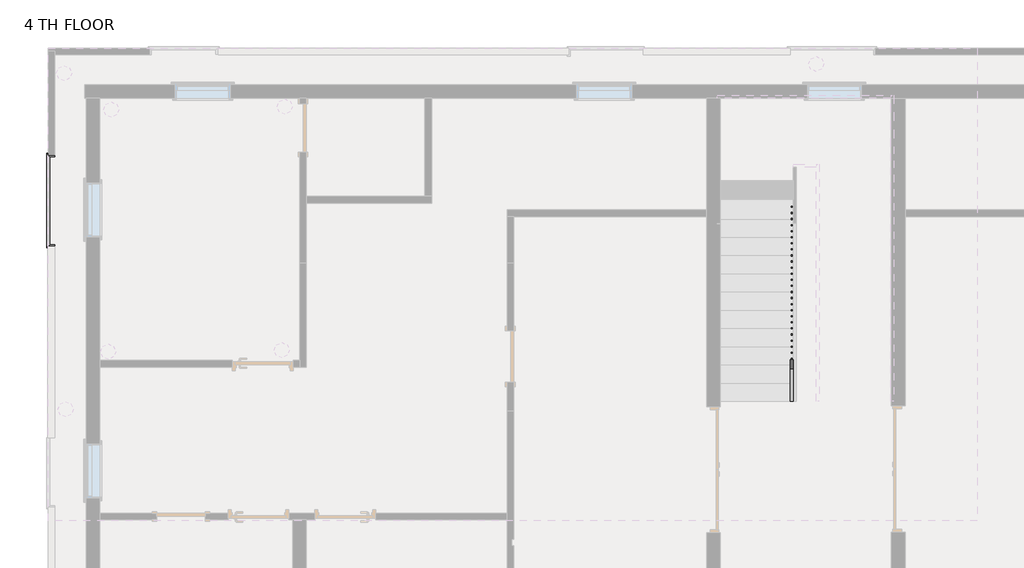
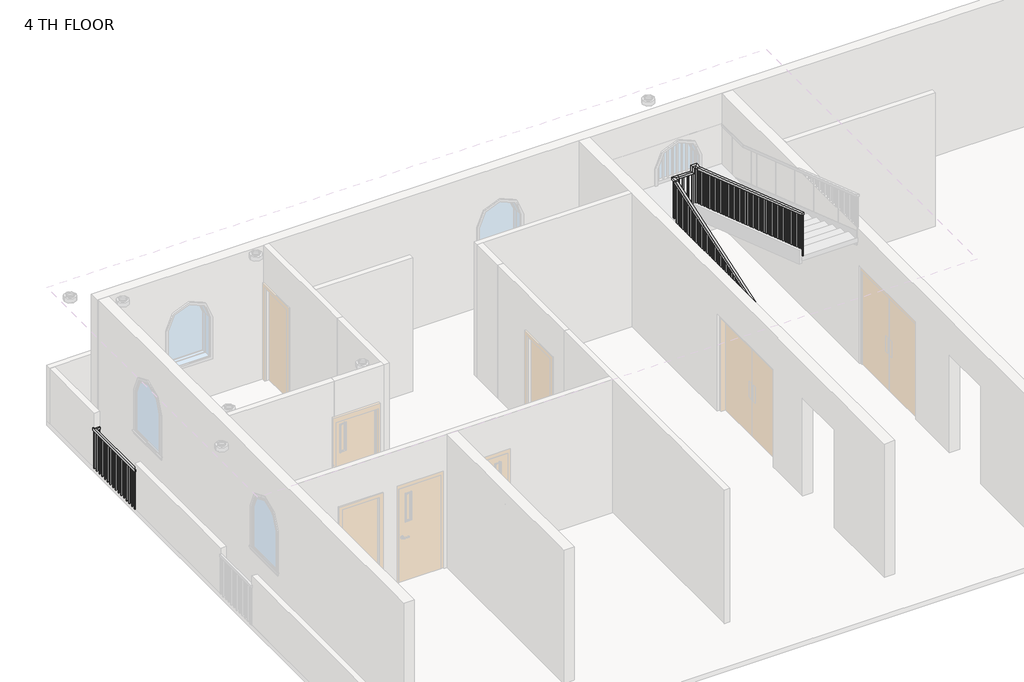
# One storey, part 4 of 7: 2 railings.
"""IFC4 building model written with IfcOpenShell, lengths in millimetres."""

from ifc_helpers import new_model, si_unit, frame, origin, place, context, project, spatial, polyline, outline, extrude, faceted_brep, element, save

model = new_model("IFC4")

# Units and contexts
model_context = context("Model", 3, world=origin())
ifc_project = project(units=[si_unit("LENGTHUNIT", "METRE", prefix="MILLI")], contexts=[model_context])

# Site, building, storey
site = spatial("IfcSite", under=ifc_project)
building = spatial("IfcBuilding", under=site)
storey = spatial("IfcBuildingStorey", under=building, Name="4 TH FLOOR", Elevation=12801.6)

# Railings
placement = place(None, origin())
element("IfcRailing", 1, ObjectType="Handrail - Rectangular", at=placement, inside=storey, context=model_context, shape_type="SolidModel", body=[
    faceted_brep([(-680.3987998, 2564.5067329, 13819.4142857), (-680.3987998, 2564.5067329, 13765.7699957), (-629.5987998, 2564.5067329, 13765.7699957), (-629.5987998, 2564.5067329, 13819.4142857), (-680.3987998, 6450.7067329, 15137.9464286), (-680.3987998, 6501.5067329, 15101.5378529), (-629.5987998, 6501.5067329, 15101.5378529), (-629.5987998, 6450.7067329, 15137.9464286), (-553.3987998, 6577.7067329, 15113.0), (-553.3987998, 6577.7067329, 15163.8), (-273.9987915, 6577.7067329, 15163.8), (-223.1987915, 6577.7067329, 15113.0), (-553.3987998, 6526.9067329, 15113.0), (-223.1987915, 6526.9067329, 15113.0), (-553.3987998, 6526.9067329, 15163.8), (-273.9987915, 6526.9067329, 15163.8), (-146.9987915, 2564.5067329, 16611.6), (-197.7987915, 2564.5067329, 16611.6), (-197.7987915, 2564.5067329, 16557.95571), (-146.9987915, 2564.5067329, 16557.95571), (-146.9987915, 6442.3235624, 15242.2678571), (-146.9987915, 6450.7067329, 15293.0678571), (-197.7987915, 6442.3235624, 15242.2678571), (-197.7987915, 6450.7067329, 15293.0678571), (-680.3987998, 6450.7067329, 15163.8), (-680.3987998, 6501.5067329, 15113.0), (-629.5987998, 6501.5067329, 15113.0), (-629.5987998, 6450.7067329, 15163.8), (-680.3987998, 6577.7067329, 15163.8), (-680.3987998, 6577.7067329, 15113.0), (-629.5987998, 6526.9067329, 15113.0), (-629.5987998, 6526.9067329, 15163.8), (-273.9987915, 6577.7067329, 15293.0678571), (-223.1987915, 6577.7067329, 15242.2678571), (-223.1987915, 6526.9067329, 15242.2678571), (-273.9987915, 6526.9067329, 15293.0678571), (-146.9987915, 6577.7067329, 15293.0678571), (-146.9987915, 6577.7067329, 15242.2678571), (-197.7987915, 6526.9067329, 15242.2678571), (-197.7987915, 6526.9067329, 15293.0678571)], [[[0, 1, 2, 3]], [[1, 0, 4, 5]], [[2, 1, 5, 6]], [[3, 2, 6, 7]], [[0, 3, 7, 4]], [[8, 9, 10, 11]], [[12, 8, 11, 13]], [[14, 12, 13, 15]], [[9, 14, 15, 10]], [[16, 17, 18, 19]], [[20, 21, 16, 19]], [[22, 20, 19, 18]], [[23, 22, 18, 17]], [[21, 23, 17, 16]], [[5, 4, 24, 25]], [[6, 5, 25, 26]], [[7, 6, 26, 27]], [[4, 7, 27, 24]], [[25, 24, 28, 29]], [[26, 25, 29, 30]], [[27, 26, 30, 31]], [[24, 27, 31, 28]], [[29, 28, 9, 8]], [[30, 29, 8, 12]], [[31, 30, 12, 14]], [[28, 31, 14, 9]], [[11, 10, 32, 33]], [[13, 11, 33, 34]], [[15, 13, 34, 35]], [[10, 15, 35, 32]], [[33, 32, 36, 37]], [[34, 33, 37, 38]], [[35, 34, 38, 39]], [[32, 35, 39, 36]], [[37, 36, 21, 20]], [[38, 37, 20, 22]], [[39, 38, 22, 23]], [[36, 39, 23, 21]]]),
    extrude(outline(polyline([(2580.3817329, 16552.5695493), (2599.4317329, 16546.1061565), (2599.4317329, 15593.7857143), (2580.3817329, 15593.7857143), (2580.3817329, 16552.5695493)])), frame((-181.9237915, 0.0, 0.0), z_axis=(1.0, 0.0, 0.0), x_axis=(0.0, 1.0, 0.0)), (0.0, 0.0, 1.0), 19.05),
    extrude(outline(polyline([(2681.9817329, 16518.0981207), (2701.0317329, 16511.6347279), (2701.0317329, 15593.7857143), (2681.9817329, 15593.7857143), (2681.9817329, 16518.0981207)])), frame((-181.9237915, 0.0, 0.0), z_axis=(1.0, 0.0, 0.0), x_axis=(0.0, 1.0, 0.0)), (0.0, 0.0, 1.0), 19.05),
    extrude(outline(polyline([(2783.5817329, 16483.6266922), (2802.6317329, 16477.1632993), (2802.6317329, 15593.7857143), (2783.5817329, 15593.7857143), (2783.5817329, 16483.6266922)])), frame((-181.9237915, 0.0, 0.0), z_axis=(1.0, 0.0, 0.0), x_axis=(0.0, 1.0, 0.0)), (0.0, 0.0, 1.0), 19.05),
    extrude(outline(polyline([(2885.1817329, 16449.1552636), (2904.2317329, 16442.6918707), (2904.2317329, 15490.3714286), (2885.1817329, 15490.3714286), (2885.1817329, 16449.1552636)])), frame((-181.9237915, 0.0, 0.0), z_axis=(1.0, 0.0, 0.0), x_axis=(0.0, 1.0, 0.0)), (0.0, 0.0, 1.0), 19.05),
    extrude(outline(polyline([(2986.7817329, 16414.683835), (3005.8317329, 16408.2204422), (3005.8317329, 15490.3714286), (2986.7817329, 15490.3714286), (2986.7817329, 16414.683835)])), frame((-181.9237915, 0.0, 0.0), z_axis=(1.0, 0.0, 0.0), x_axis=(0.0, 1.0, 0.0)), (0.0, 0.0, 1.0), 19.05),
    extrude(outline(polyline([(3088.3817329, 16380.2124065), (3107.4317329, 16373.7490136), (3107.4317329, 15490.3714286), (3088.3817329, 15490.3714286), (3088.3817329, 16380.2124065)])), frame((-181.9237915, 0.0, 0.0), z_axis=(1.0, 0.0, 0.0), x_axis=(0.0, 1.0, 0.0)), (0.0, 0.0, 1.0), 19.05),
    extrude(outline(polyline([(3189.9817329, 16345.7409779), (3209.0317329, 16339.277585), (3209.0317329, 15386.9571429), (3189.9817329, 15386.9571429), (3189.9817329, 16345.7409779)])), frame((-181.9237915, 0.0, 0.0), z_axis=(1.0, 0.0, 0.0), x_axis=(0.0, 1.0, 0.0)), (0.0, 0.0, 1.0), 19.05),
    extrude(outline(polyline([(3291.5817329, 16311.2695493), (3310.6317329, 16304.8061565), (3310.6317329, 15386.9571429), (3291.5817329, 15386.9571429), (3291.5817329, 16311.2695493)])), frame((-181.9237915, 0.0, 0.0), z_axis=(1.0, 0.0, 0.0), x_axis=(0.0, 1.0, 0.0)), (0.0, 0.0, 1.0), 19.05),
    extrude(outline(polyline([(3393.1817329, 16276.7981207), (3412.2317329, 16270.3347279), (3412.2317329, 15386.9571429), (3393.1817329, 15386.9571429), (3393.1817329, 16276.7981207)])), frame((-181.9237915, 0.0, 0.0), z_axis=(1.0, 0.0, 0.0), x_axis=(0.0, 1.0, 0.0)), (0.0, 0.0, 1.0), 19.05),
    extrude(outline(polyline([(3494.7817329, 16242.3266922), (3513.8317329, 16235.8632993), (3513.8317329, 15283.5428571), (3494.7817329, 15283.5428571), (3494.7817329, 16242.3266922)])), frame((-181.9237915, 0.0, 0.0), z_axis=(1.0, 0.0, 0.0), x_axis=(0.0, 1.0, 0.0)), (0.0, 0.0, 1.0), 19.05),
    extrude(outline(polyline([(3596.3817329, 16207.8552636), (3615.4317329, 16201.3918707), (3615.4317329, 15283.5428571), (3596.3817329, 15283.5428571), (3596.3817329, 16207.8552636)])), frame((-181.9237915, 0.0, 0.0), z_axis=(1.0, 0.0, 0.0), x_axis=(0.0, 1.0, 0.0)), (0.0, 0.0, 1.0), 19.05),
    extrude(outline(polyline([(3697.9817329, 16173.383835), (3717.0317329, 16166.9204422), (3717.0317329, 15283.5428571), (3697.9817329, 15283.5428571), (3697.9817329, 16173.383835)])), frame((-181.9237915, 0.0, 0.0), z_axis=(1.0, 0.0, 0.0), x_axis=(0.0, 1.0, 0.0)), (0.0, 0.0, 1.0), 19.05),
    extrude(outline(polyline([(3799.5817329, 16138.9124065), (3818.6317329, 16132.4490136), (3818.6317329, 15180.1285714), (3799.5817329, 15180.1285714), (3799.5817329, 16138.9124065)])), frame((-181.9237915, 0.0, 0.0), z_axis=(1.0, 0.0, 0.0), x_axis=(0.0, 1.0, 0.0)), (0.0, 0.0, 1.0), 19.05),
    extrude(outline(polyline([(3901.1817329, 16104.4409779), (3920.2317329, 16097.977585), (3920.2317329, 15180.1285714), (3901.1817329, 15180.1285714), (3901.1817329, 16104.4409779)])), frame((-181.9237915, 0.0, 0.0), z_axis=(1.0, 0.0, 0.0), x_axis=(0.0, 1.0, 0.0)), (0.0, 0.0, 1.0), 19.05),
    extrude(outline(polyline([(4002.7817329, 16069.9695493), (4021.8317329, 16063.5061565), (4021.8317329, 15180.1285714), (4002.7817329, 15180.1285714), (4002.7817329, 16069.9695493)])), frame((-181.9237915, 0.0, 0.0), z_axis=(1.0, 0.0, 0.0), x_axis=(0.0, 1.0, 0.0)), (0.0, 0.0, 1.0), 19.05),
    extrude(outline(polyline([(4104.3817329, 16035.4981207), (4123.4317329, 16029.0347279), (4123.4317329, 15076.7142857), (4104.3817329, 15076.7142857), (4104.3817329, 16035.4981207)])), frame((-181.9237915, 0.0, 0.0), z_axis=(1.0, 0.0, 0.0), x_axis=(0.0, 1.0, 0.0)), (0.0, 0.0, 1.0), 19.05),
    extrude(outline(polyline([(4205.9817329, 16001.0266922), (4225.0317329, 15994.5632993), (4225.0317329, 15076.7142857), (4205.9817329, 15076.7142857), (4205.9817329, 16001.0266922)])), frame((-181.9237915, 0.0, 0.0), z_axis=(1.0, 0.0, 0.0), x_axis=(0.0, 1.0, 0.0)), (0.0, 0.0, 1.0), 19.05),
    extrude(outline(polyline([(4307.5817329, 15966.5552636), (4326.6317329, 15960.0918707), (4326.6317329, 15076.7142857), (4307.5817329, 15076.7142857), (4307.5817329, 15966.5552636)])), frame((-181.9237915, 0.0, 0.0), z_axis=(1.0, 0.0, 0.0), x_axis=(0.0, 1.0, 0.0)), (0.0, 0.0, 1.0), 19.05),
    extrude(outline(polyline([(4409.1817329, 15932.083835), (4428.2317329, 15925.6204422), (4428.2317329, 14973.3), (4409.1817329, 14973.3), (4409.1817329, 15932.083835)])), frame((-181.9237915, 0.0, 0.0), z_axis=(1.0, 0.0, 0.0), x_axis=(0.0, 1.0, 0.0)), (0.0, 0.0, 1.0), 19.05),
    extrude(outline(polyline([(4510.7817329, 15897.6124065), (4529.8317329, 15891.1490136), (4529.8317329, 14973.3), (4510.7817329, 14973.3), (4510.7817329, 15897.6124065)])), frame((-181.9237915, 0.0, 0.0), z_axis=(1.0, 0.0, 0.0), x_axis=(0.0, 1.0, 0.0)), (0.0, 0.0, 1.0), 19.05),
    extrude(outline(polyline([(4612.3817329, 15863.1409779), (4631.4317329, 15856.677585), (4631.4317329, 14973.3), (4612.3817329, 14973.3), (4612.3817329, 15863.1409779)])), frame((-181.9237915, 0.0, 0.0), z_axis=(1.0, 0.0, 0.0), x_axis=(0.0, 1.0, 0.0)), (0.0, 0.0, 1.0), 19.05),
    extrude(outline(polyline([(4713.9817329, 15828.6695493), (4733.0317329, 15822.2061565), (4733.0317329, 14869.8857143), (4713.9817329, 14869.8857143), (4713.9817329, 15828.6695493)])), frame((-181.9237915, 0.0, 0.0), z_axis=(1.0, 0.0, 0.0), x_axis=(0.0, 1.0, 0.0)), (0.0, 0.0, 1.0), 19.05),
    extrude(outline(polyline([(4815.5817329, 15794.1981207), (4834.6317329, 15787.7347279), (4834.6317329, 14869.8857143), (4815.5817329, 14869.8857143), (4815.5817329, 15794.1981207)])), frame((-181.9237915, 0.0, 0.0), z_axis=(1.0, 0.0, 0.0), x_axis=(0.0, 1.0, 0.0)), (0.0, 0.0, 1.0), 19.05),
    extrude(outline(polyline([(4917.1817329, 15759.7266922), (4936.2317329, 15753.2632993), (4936.2317329, 14869.8857143), (4917.1817329, 14869.8857143), (4917.1817329, 15759.7266922)])), frame((-181.9237915, 0.0, 0.0), z_axis=(1.0, 0.0, 0.0), x_axis=(0.0, 1.0, 0.0)), (0.0, 0.0, 1.0), 19.05),
    extrude(outline(polyline([(5018.7817329, 15725.2552636), (5037.8317329, 15718.7918707), (5037.8317329, 14766.4714286), (5018.7817329, 14766.4714286), (5018.7817329, 15725.2552636)])), frame((-181.9237915, 0.0, 0.0), z_axis=(1.0, 0.0, 0.0), x_axis=(0.0, 1.0, 0.0)), (0.0, 0.0, 1.0), 19.05),
    extrude(outline(polyline([(5120.3817329, 15690.783835), (5139.4317329, 15684.3204422), (5139.4317329, 14766.4714286), (5120.3817329, 14766.4714286), (5120.3817329, 15690.783835)])), frame((-181.9237915, 0.0, 0.0), z_axis=(1.0, 0.0, 0.0), x_axis=(0.0, 1.0, 0.0)), (0.0, 0.0, 1.0), 19.05),
    extrude(outline(polyline([(5221.9817329, 15656.3124065), (5241.0317329, 15649.8490136), (5241.0317329, 14766.4714286), (5221.9817329, 14766.4714286), (5221.9817329, 15656.3124065)])), frame((-181.9237915, 0.0, 0.0), z_axis=(1.0, 0.0, 0.0), x_axis=(0.0, 1.0, 0.0)), (0.0, 0.0, 1.0), 19.05),
    extrude(outline(polyline([(5323.5817329, 15621.8409779), (5342.6317329, 15615.377585), (5342.6317329, 14663.0571429), (5323.5817329, 14663.0571429), (5323.5817329, 15621.8409779)])), frame((-181.9237915, 0.0, 0.0), z_axis=(1.0, 0.0, 0.0), x_axis=(0.0, 1.0, 0.0)), (0.0, 0.0, 1.0), 19.05),
    extrude(outline(polyline([(5425.1817329, 15587.3695493), (5444.2317329, 15580.9061565), (5444.2317329, 14663.0571429), (5425.1817329, 14663.0571429), (5425.1817329, 15587.3695493)])), frame((-181.9237915, 0.0, 0.0), z_axis=(1.0, 0.0, 0.0), x_axis=(0.0, 1.0, 0.0)), (0.0, 0.0, 1.0), 19.05),
    extrude(outline(polyline([(5526.7817329, 15552.8981207), (5545.8317329, 15546.4347279), (5545.8317329, 14663.0571429), (5526.7817329, 14663.0571429), (5526.7817329, 15552.8981207)])), frame((-181.9237915, 0.0, 0.0), z_axis=(1.0, 0.0, 0.0), x_axis=(0.0, 1.0, 0.0)), (0.0, 0.0, 1.0), 19.05),
    extrude(outline(polyline([(5628.3817329, 15518.4266922), (5647.4317329, 15511.9632993), (5647.4317329, 14559.6428571), (5628.3817329, 14559.6428571), (5628.3817329, 15518.4266922)])), frame((-181.9237915, 0.0, 0.0), z_axis=(1.0, 0.0, 0.0), x_axis=(0.0, 1.0, 0.0)), (0.0, 0.0, 1.0), 19.05),
    extrude(outline(polyline([(5729.9817329, 15483.9552636), (5749.0317329, 15477.4918707), (5749.0317329, 14559.6428571), (5729.9817329, 14559.6428571), (5729.9817329, 15483.9552636)])), frame((-181.9237915, 0.0, 0.0), z_axis=(1.0, 0.0, 0.0), x_axis=(0.0, 1.0, 0.0)), (0.0, 0.0, 1.0), 19.05),
    extrude(outline(polyline([(5831.5817329, 15449.483835), (5850.6317329, 15443.0204422), (5850.6317329, 14559.6428571), (5831.5817329, 14559.6428571), (5831.5817329, 15449.483835)])), frame((-181.9237915, 0.0, 0.0), z_axis=(1.0, 0.0, 0.0), x_axis=(0.0, 1.0, 0.0)), (0.0, 0.0, 1.0), 19.05),
    extrude(outline(polyline([(5933.1817329, 15415.0124065), (5952.2317329, 15408.5490136), (5952.2317329, 14456.2285714), (5933.1817329, 14456.2285714), (5933.1817329, 15415.0124065)])), frame((-181.9237915, 0.0, 0.0), z_axis=(1.0, 0.0, 0.0), x_axis=(0.0, 1.0, 0.0)), (0.0, 0.0, 1.0), 19.05),
    extrude(outline(polyline([(6034.7817329, 15380.5409779), (6053.8317329, 15374.077585), (6053.8317329, 14456.2285714), (6034.7817329, 14456.2285714), (6034.7817329, 15380.5409779)])), frame((-181.9237915, 0.0, 0.0), z_axis=(1.0, 0.0, 0.0), x_axis=(0.0, 1.0, 0.0)), (0.0, 0.0, 1.0), 19.05),
    extrude(outline(polyline([(6136.3817329, 15346.0695493), (6155.4317329, 15339.6061565), (6155.4317329, 14456.2285714), (6136.3817329, 14456.2285714), (6136.3817329, 15346.0695493)])), frame((-181.9237915, 0.0, 0.0), z_axis=(1.0, 0.0, 0.0), x_axis=(0.0, 1.0, 0.0)), (0.0, 0.0, 1.0), 19.05),
    extrude(outline(polyline([(6237.9817329, 15311.5981207), (6257.0317329, 15305.1347279), (6257.0317329, 14352.8142857), (6237.9817329, 14352.8142857), (6237.9817329, 15311.5981207)])), frame((-181.9237915, 0.0, 0.0), z_axis=(1.0, 0.0, 0.0), x_axis=(0.0, 1.0, 0.0)), (0.0, 0.0, 1.0), 19.05),
    extrude(outline(polyline([(6339.5817329, 15277.1266922), (6358.6317329, 15270.6632993), (6358.6317329, 14352.8142857), (6339.5817329, 14352.8142857), (6339.5817329, 15277.1266922)])), frame((-181.9237915, 0.0, 0.0), z_axis=(1.0, 0.0, 0.0), x_axis=(0.0, 1.0, 0.0)), (0.0, 0.0, 1.0), 19.05),
    extrude(outline(polyline([(6441.1817329, 15242.6552636), (6460.2317329, 15236.1918707), (6460.2317329, 14352.8142857), (6441.1817329, 14352.8142857), (6441.1817329, 15242.6552636)])), frame((-181.9237915, 0.0, 0.0), z_axis=(1.0, 0.0, 0.0), x_axis=(0.0, 1.0, 0.0)), (0.0, 0.0, 1.0), 19.05),
    extrude(outline(polyline([(-258.1237998, 6542.7817329), (-258.1237998, 6561.8317329), (-239.0737998, 6561.8317329), (-239.0737998, 6542.7817329), (-258.1237998, 6542.7817329)])), frame((0.0, 0.0, 14249.4), z_axis=(0.0, 0.0, 1.0), x_axis=(1.0, 0.0, 0.0)), (0.0, 0.0, 1.0), 992.8678571),
    extrude(outline(polyline([(-359.7237998, 6542.7817329), (-359.7237998, 6561.8317329), (-340.6737998, 6561.8317329), (-340.6737998, 6542.7817329), (-359.7237998, 6542.7817329)])), frame((0.0, 0.0, 14249.4), z_axis=(0.0, 0.0, 1.0), x_axis=(1.0, 0.0, 0.0)), (0.0, 0.0, 1.0), 863.6),
    extrude(outline(polyline([(-461.3237998, 6542.7817329), (-461.3237998, 6561.8317329), (-442.2737998, 6561.8317329), (-442.2737998, 6542.7817329), (-461.3237998, 6542.7817329)])), frame((0.0, 0.0, 14249.4), z_axis=(0.0, 0.0, 1.0), x_axis=(1.0, 0.0, 0.0)), (0.0, 0.0, 1.0), 863.6),
    extrude(outline(polyline([(-562.9237998, 6542.7817329), (-562.9237998, 6561.8317329), (-543.8737998, 6561.8317329), (-543.8737998, 6542.7817329), (-562.9237998, 6542.7817329)])), frame((0.0, 0.0, 14249.4), z_axis=(0.0, 0.0, 1.0), x_axis=(1.0, 0.0, 0.0)), (0.0, 0.0, 1.0), 863.6),
    extrude(outline(polyline([(-645.4737998, 6517.3817329), (-664.5237998, 6517.3817329), (-664.5237998, 6536.4317329), (-645.4737998, 6536.4317329), (-645.4737998, 6517.3817329)])), frame((0.0, 0.0, 14249.4), z_axis=(0.0, 0.0, 1.0), x_axis=(1.0, 0.0, 0.0)), (0.0, 0.0, 1.0), 863.6),
    extrude(outline(polyline([(6415.7817329, 15072.452585), (6434.8317329, 15078.9159779), (6434.8317329, 14145.9857143), (6415.7817329, 14145.9857143), (6415.7817329, 15072.452585)])), frame((-664.5237998, 0.0, 0.0), z_axis=(1.0, 0.0, 0.0), x_axis=(0.0, 1.0, 0.0)), (0.0, 0.0, 1.0), 19.05),
    extrude(outline(polyline([(6314.1817329, 15037.9811565), (6333.2317329, 15044.4445493), (6333.2317329, 14145.9857143), (6314.1817329, 14145.9857143), (6314.1817329, 15037.9811565)])), frame((-664.5237998, 0.0, 0.0), z_axis=(1.0, 0.0, 0.0), x_axis=(0.0, 1.0, 0.0)), (0.0, 0.0, 1.0), 19.05),
    extrude(outline(polyline([(6212.5817329, 15003.5097279), (6231.6317329, 15009.9731207), (6231.6317329, 14145.9857143), (6212.5817329, 14145.9857143), (6212.5817329, 15003.5097279)])), frame((-664.5237998, 0.0, 0.0), z_axis=(1.0, 0.0, 0.0), x_axis=(0.0, 1.0, 0.0)), (0.0, 0.0, 1.0), 19.05),
    extrude(outline(polyline([(6110.9817329, 14969.0382993), (6130.0317329, 14975.5016922), (6130.0317329, 14042.5714286), (6110.9817329, 14042.5714286), (6110.9817329, 14969.0382993)])), frame((-664.5237998, 0.0, 0.0), z_axis=(1.0, 0.0, 0.0), x_axis=(0.0, 1.0, 0.0)), (0.0, 0.0, 1.0), 19.05),
    extrude(outline(polyline([(6009.3817329, 14934.5668707), (6028.4317329, 14941.0302636), (6028.4317329, 14042.5714286), (6009.3817329, 14042.5714286), (6009.3817329, 14934.5668707)])), frame((-664.5237998, 0.0, 0.0), z_axis=(1.0, 0.0, 0.0), x_axis=(0.0, 1.0, 0.0)), (0.0, 0.0, 1.0), 19.05),
    extrude(outline(polyline([(5907.7817329, 14900.0954422), (5926.8317329, 14906.558835), (5926.8317329, 14042.5714286), (5907.7817329, 14042.5714286), (5907.7817329, 14900.0954422)])), frame((-664.5237998, 0.0, 0.0), z_axis=(1.0, 0.0, 0.0), x_axis=(0.0, 1.0, 0.0)), (0.0, 0.0, 1.0), 19.05),
    extrude(outline(polyline([(5806.1817329, 14865.6240136), (5825.2317329, 14872.0874065), (5825.2317329, 13939.1571429), (5806.1817329, 13939.1571429), (5806.1817329, 14865.6240136)])), frame((-664.5237998, 0.0, 0.0), z_axis=(1.0, 0.0, 0.0), x_axis=(0.0, 1.0, 0.0)), (0.0, 0.0, 1.0), 19.05),
    extrude(outline(polyline([(5704.5817329, 14831.152585), (5723.6317329, 14837.6159779), (5723.6317329, 13939.1571429), (5704.5817329, 13939.1571429), (5704.5817329, 14831.152585)])), frame((-664.5237998, 0.0, 0.0), z_axis=(1.0, 0.0, 0.0), x_axis=(0.0, 1.0, 0.0)), (0.0, 0.0, 1.0), 19.05),
    extrude(outline(polyline([(5602.9817329, 14796.6811565), (5622.0317329, 14803.1445493), (5622.0317329, 13939.1571429), (5602.9817329, 13939.1571429), (5602.9817329, 14796.6811565)])), frame((-664.5237998, 0.0, 0.0), z_axis=(1.0, 0.0, 0.0), x_axis=(0.0, 1.0, 0.0)), (0.0, 0.0, 1.0), 19.05),
    extrude(outline(polyline([(5501.3817329, 14762.2097279), (5520.4317329, 14768.6731207), (5520.4317329, 13835.7428571), (5501.3817329, 13835.7428571), (5501.3817329, 14762.2097279)])), frame((-664.5237998, 0.0, 0.0), z_axis=(1.0, 0.0, 0.0), x_axis=(0.0, 1.0, 0.0)), (0.0, 0.0, 1.0), 19.05),
    extrude(outline(polyline([(5399.7817329, 14727.7382993), (5418.8317329, 14734.2016922), (5418.8317329, 13835.7428571), (5399.7817329, 13835.7428571), (5399.7817329, 14727.7382993)])), frame((-664.5237998, 0.0, 0.0), z_axis=(1.0, 0.0, 0.0), x_axis=(0.0, 1.0, 0.0)), (0.0, 0.0, 1.0), 19.05),
    extrude(outline(polyline([(5298.1817329, 14693.2668707), (5317.2317329, 14699.7302636), (5317.2317329, 13835.7428571), (5298.1817329, 13835.7428571), (5298.1817329, 14693.2668707)])), frame((-664.5237998, 0.0, 0.0), z_axis=(1.0, 0.0, 0.0), x_axis=(0.0, 1.0, 0.0)), (0.0, 0.0, 1.0), 19.05),
    extrude(outline(polyline([(5196.5817329, 14658.7954422), (5215.6317329, 14665.258835), (5215.6317329, 13732.3285714), (5196.5817329, 13732.3285714), (5196.5817329, 14658.7954422)])), frame((-664.5237998, 0.0, 0.0), z_axis=(1.0, 0.0, 0.0), x_axis=(0.0, 1.0, 0.0)), (0.0, 0.0, 1.0), 19.05),
    extrude(outline(polyline([(5094.9817329, 14624.3240136), (5114.0317329, 14630.7874065), (5114.0317329, 13732.3285714), (5094.9817329, 13732.3285714), (5094.9817329, 14624.3240136)])), frame((-664.5237998, 0.0, 0.0), z_axis=(1.0, 0.0, 0.0), x_axis=(0.0, 1.0, 0.0)), (0.0, 0.0, 1.0), 19.05),
    extrude(outline(polyline([(4993.3817329, 14589.852585), (5012.4317329, 14596.3159779), (5012.4317329, 13732.3285714), (4993.3817329, 13732.3285714), (4993.3817329, 14589.852585)])), frame((-664.5237998, 0.0, 0.0), z_axis=(1.0, 0.0, 0.0), x_axis=(0.0, 1.0, 0.0)), (0.0, 0.0, 1.0), 19.05),
    extrude(outline(polyline([(4891.7817329, 14555.3811565), (4910.8317329, 14561.8445493), (4910.8317329, 13628.9142857), (4891.7817329, 13628.9142857), (4891.7817329, 14555.3811565)])), frame((-664.5237998, 0.0, 0.0), z_axis=(1.0, 0.0, 0.0), x_axis=(0.0, 1.0, 0.0)), (0.0, 0.0, 1.0), 19.05),
    extrude(outline(polyline([(4790.1817329, 14520.9097279), (4809.2317329, 14527.3731207), (4809.2317329, 13628.9142857), (4790.1817329, 13628.9142857), (4790.1817329, 14520.9097279)])), frame((-664.5237998, 0.0, 0.0), z_axis=(1.0, 0.0, 0.0), x_axis=(0.0, 1.0, 0.0)), (0.0, 0.0, 1.0), 19.05),
    extrude(outline(polyline([(4688.5817329, 14486.4382993), (4707.6317329, 14492.9016922), (4707.6317329, 13628.9142857), (4688.5817329, 13628.9142857), (4688.5817329, 14486.4382993)])), frame((-664.5237998, 0.0, 0.0), z_axis=(1.0, 0.0, 0.0), x_axis=(0.0, 1.0, 0.0)), (0.0, 0.0, 1.0), 19.05),
    extrude(outline(polyline([(4586.9817329, 14451.9668707), (4606.0317329, 14458.4302636), (4606.0317329, 13525.5), (4586.9817329, 13525.5), (4586.9817329, 14451.9668707)])), frame((-664.5237998, 0.0, 0.0), z_axis=(1.0, 0.0, 0.0), x_axis=(0.0, 1.0, 0.0)), (0.0, 0.0, 1.0), 19.05),
    extrude(outline(polyline([(4485.3817329, 14417.4954422), (4504.4317329, 14423.958835), (4504.4317329, 13525.5), (4485.3817329, 13525.5), (4485.3817329, 14417.4954422)])), frame((-664.5237998, 0.0, 0.0), z_axis=(1.0, 0.0, 0.0), x_axis=(0.0, 1.0, 0.0)), (0.0, 0.0, 1.0), 19.05),
    extrude(outline(polyline([(4383.7817329, 14383.0240136), (4402.8317329, 14389.4874065), (4402.8317329, 13525.5), (4383.7817329, 13525.5), (4383.7817329, 14383.0240136)])), frame((-664.5237998, 0.0, 0.0), z_axis=(1.0, 0.0, 0.0), x_axis=(0.0, 1.0, 0.0)), (0.0, 0.0, 1.0), 19.05),
    extrude(outline(polyline([(4282.1817329, 14348.552585), (4301.2317329, 14355.0159779), (4301.2317329, 13422.0857143), (4282.1817329, 13422.0857143), (4282.1817329, 14348.552585)])), frame((-664.5237998, 0.0, 0.0), z_axis=(1.0, 0.0, 0.0), x_axis=(0.0, 1.0, 0.0)), (0.0, 0.0, 1.0), 19.05),
    extrude(outline(polyline([(4180.5817329, 14314.0811565), (4199.6317329, 14320.5445493), (4199.6317329, 13422.0857143), (4180.5817329, 13422.0857143), (4180.5817329, 14314.0811565)])), frame((-664.5237998, 0.0, 0.0), z_axis=(1.0, 0.0, 0.0), x_axis=(0.0, 1.0, 0.0)), (0.0, 0.0, 1.0), 19.05),
    extrude(outline(polyline([(4078.9817329, 14279.6097279), (4098.0317329, 14286.0731207), (4098.0317329, 13422.0857143), (4078.9817329, 13422.0857143), (4078.9817329, 14279.6097279)])), frame((-664.5237998, 0.0, 0.0), z_axis=(1.0, 0.0, 0.0), x_axis=(0.0, 1.0, 0.0)), (0.0, 0.0, 1.0), 19.05),
    extrude(outline(polyline([(3977.3817329, 14245.1382993), (3996.4317329, 14251.6016922), (3996.4317329, 13318.6714286), (3977.3817329, 13318.6714286), (3977.3817329, 14245.1382993)])), frame((-664.5237998, 0.0, 0.0), z_axis=(1.0, 0.0, 0.0), x_axis=(0.0, 1.0, 0.0)), (0.0, 0.0, 1.0), 19.05),
    extrude(outline(polyline([(3875.7817329, 14210.6668707), (3894.8317329, 14217.1302636), (3894.8317329, 13318.6714286), (3875.7817329, 13318.6714286), (3875.7817329, 14210.6668707)])), frame((-664.5237998, 0.0, 0.0), z_axis=(1.0, 0.0, 0.0), x_axis=(0.0, 1.0, 0.0)), (0.0, 0.0, 1.0), 19.05),
    extrude(outline(polyline([(3774.1817329, 14176.1954422), (3793.2317329, 14182.658835), (3793.2317329, 13318.6714286), (3774.1817329, 13318.6714286), (3774.1817329, 14176.1954422)])), frame((-664.5237998, 0.0, 0.0), z_axis=(1.0, 0.0, 0.0), x_axis=(0.0, 1.0, 0.0)), (0.0, 0.0, 1.0), 19.05),
    extrude(outline(polyline([(3672.5817329, 14141.7240136), (3691.6317329, 14148.1874065), (3691.6317329, 13215.2571429), (3672.5817329, 13215.2571429), (3672.5817329, 14141.7240136)])), frame((-664.5237998, 0.0, 0.0), z_axis=(1.0, 0.0, 0.0), x_axis=(0.0, 1.0, 0.0)), (0.0, 0.0, 1.0), 19.05),
    extrude(outline(polyline([(3570.9817329, 14107.252585), (3590.0317329, 14113.7159779), (3590.0317329, 13215.2571429), (3570.9817329, 13215.2571429), (3570.9817329, 14107.252585)])), frame((-664.5237998, 0.0, 0.0), z_axis=(1.0, 0.0, 0.0), x_axis=(0.0, 1.0, 0.0)), (0.0, 0.0, 1.0), 19.05),
    extrude(outline(polyline([(3469.3817329, 14072.7811565), (3488.4317329, 14079.2445493), (3488.4317329, 13215.2571429), (3469.3817329, 13215.2571429), (3469.3817329, 14072.7811565)])), frame((-664.5237998, 0.0, 0.0), z_axis=(1.0, 0.0, 0.0), x_axis=(0.0, 1.0, 0.0)), (0.0, 0.0, 1.0), 19.05),
    extrude(outline(polyline([(3367.7817329, 14038.3097279), (3386.8317329, 14044.7731207), (3386.8317329, 13111.8428571), (3367.7817329, 13111.8428571), (3367.7817329, 14038.3097279)])), frame((-664.5237998, 0.0, 0.0), z_axis=(1.0, 0.0, 0.0), x_axis=(0.0, 1.0, 0.0)), (0.0, 0.0, 1.0), 19.05),
    extrude(outline(polyline([(3266.1817329, 14003.8382993), (3285.2317329, 14010.3016922), (3285.2317329, 13111.8428571), (3266.1817329, 13111.8428571), (3266.1817329, 14003.8382993)])), frame((-664.5237998, 0.0, 0.0), z_axis=(1.0, 0.0, 0.0), x_axis=(0.0, 1.0, 0.0)), (0.0, 0.0, 1.0), 19.05),
    extrude(outline(polyline([(3164.5817329, 13969.3668707), (3183.6317329, 13975.8302636), (3183.6317329, 13111.8428571), (3164.5817329, 13111.8428571), (3164.5817329, 13969.3668707)])), frame((-664.5237998, 0.0, 0.0), z_axis=(1.0, 0.0, 0.0), x_axis=(0.0, 1.0, 0.0)), (0.0, 0.0, 1.0), 19.05),
    extrude(outline(polyline([(3062.9817329, 13934.8954422), (3082.0317329, 13941.358835), (3082.0317329, 13008.4285714), (3062.9817329, 13008.4285714), (3062.9817329, 13934.8954422)])), frame((-664.5237998, 0.0, 0.0), z_axis=(1.0, 0.0, 0.0), x_axis=(0.0, 1.0, 0.0)), (0.0, 0.0, 1.0), 19.05),
    extrude(outline(polyline([(2961.3817329, 13900.4240136), (2980.4317329, 13906.8874065), (2980.4317329, 13008.4285714), (2961.3817329, 13008.4285714), (2961.3817329, 13900.4240136)])), frame((-664.5237998, 0.0, 0.0), z_axis=(1.0, 0.0, 0.0), x_axis=(0.0, 1.0, 0.0)), (0.0, 0.0, 1.0), 19.05),
    extrude(outline(polyline([(2859.7817329, 13865.952585), (2878.8317329, 13872.4159779), (2878.8317329, 13008.4285714), (2859.7817329, 13008.4285714), (2859.7817329, 13865.952585)])), frame((-664.5237998, 0.0, 0.0), z_axis=(1.0, 0.0, 0.0), x_axis=(0.0, 1.0, 0.0)), (0.0, 0.0, 1.0), 19.05),
    extrude(outline(polyline([(2758.1817329, 13831.4811565), (2777.2317329, 13837.9445493), (2777.2317329, 12905.0142857), (2758.1817329, 12905.0142857), (2758.1817329, 13831.4811565)])), frame((-664.5237998, 0.0, 0.0), z_axis=(1.0, 0.0, 0.0), x_axis=(0.0, 1.0, 0.0)), (0.0, 0.0, 1.0), 19.05),
    extrude(outline(polyline([(2656.5817329, 13797.0097279), (2675.6317329, 13803.4731207), (2675.6317329, 12905.0142857), (2656.5817329, 12905.0142857), (2656.5817329, 13797.0097279)])), frame((-664.5237998, 0.0, 0.0), z_axis=(1.0, 0.0, 0.0), x_axis=(0.0, 1.0, 0.0)), (0.0, 0.0, 1.0), 19.05),
    extrude(outline(polyline([(-181.9237915, 6542.7817329), (-181.9237915, 6561.8317329), (-162.8737915, 6561.8317329), (-162.8737915, 6542.7817329), (-181.9237915, 6542.7817329)])), frame((0.0, 0.0, 14249.4), z_axis=(0.0, 0.0, 1.0), x_axis=(1.0, 0.0, 0.0)), (0.0, 0.0, 1.0), 992.8678571),
    extrude(outline(polyline([(-645.4737998, 6542.7817329), (-664.5237998, 6542.7817329), (-664.5237998, 6561.8317329), (-645.4737998, 6561.8317329), (-645.4737998, 6542.7817329)])), frame((0.0, 0.0, 14249.4), z_axis=(0.0, 0.0, 1.0), x_axis=(1.0, 0.0, 0.0)), (0.0, 0.0, 1.0), 863.6),
    extrude(outline(polyline([(2564.5067329, 16557.95571), (2583.5567329, 16551.4923172), (2583.5567329, 15593.7857143), (2564.5067329, 15593.7857143), (2564.5067329, 16557.95571)])), frame((-181.9237915, 0.0, 0.0), z_axis=(1.0, 0.0, 0.0), x_axis=(0.0, 1.0, 0.0)), (0.0, 0.0, 1.0), 19.05),
    extrude(outline(polyline([(2564.5067329, 13765.7699957), (2583.5567329, 13772.2333886), (2583.5567329, 12905.0142857), (2564.5067329, 12905.0142857), (2564.5067329, 13765.7699957)])), frame((-664.5237998, 0.0, 0.0), z_axis=(1.0, 0.0, 0.0), x_axis=(0.0, 1.0, 0.0)), (0.0, 0.0, 1.0), 19.05),
])
element("IfcRailing", 2, ObjectType="Handrail - Rectangular", at=placement, inside=storey, context=model_context, shape_type="SolidModel", body=[
    faceted_brep([(-12973.9987925, 6656.8711337, 13716.0), (-12973.9987925, 6656.8711337, 13665.2), (-12973.9987925, 6707.6711337, 13665.2), (-12973.9987925, 6707.6711337, 13716.0), (-13062.8987925, 6656.8711337, 13716.0), (-13062.8987925, 6656.8711337, 13665.2), (-13113.6987925, 6707.6711337, 13665.2), (-13113.6987925, 6707.6711337, 13716.0), (-13062.8987925, 5180.1736362, 13716.0), (-13062.8987925, 5180.1736362, 13665.2), (-13113.6987925, 5129.3736362, 13665.2), (-13113.6987925, 5129.3736362, 13716.0), (-12973.9987925, 5180.1736362, 13716.0), (-12973.9987925, 5129.3736362, 13716.0), (-12973.9987925, 5129.3736362, 13665.2), (-12973.9987925, 5180.1736362, 13665.2)], [[[0, 1, 2, 3]], [[1, 0, 4, 5]], [[2, 1, 5, 6]], [[3, 2, 6, 7]], [[0, 3, 7, 4]], [[5, 4, 8, 9]], [[6, 5, 9, 10]], [[7, 6, 10, 11]], [[4, 7, 11, 8]], [[12, 13, 14, 15]], [[9, 8, 12, 15]], [[10, 9, 15, 14]], [[11, 10, 14, 13]], [[8, 11, 13, 12]]]),
    extrude(outline(polyline([(-12996.2237925, 5145.2486362), (-12996.2237925, 5164.2986362), (-12977.1737925, 5164.2986362), (-12977.1737925, 5145.2486362), (-12996.2237925, 5145.2486362)])), frame((0.0, 0.0, 12801.6), z_axis=(0.0, 0.0, 1.0), x_axis=(1.0, 0.0, 0.0)), (0.0, 0.0, 1.0), 863.6),
    extrude(outline(polyline([(-13097.8237925, 5167.7961337), (-13078.7737925, 5167.7961337), (-13078.7737925, 5148.7461337), (-13097.8237925, 5148.7461337), (-13097.8237925, 5167.7961337)])), frame((0.0, 0.0, 12801.6), z_axis=(0.0, 0.0, 1.0), x_axis=(1.0, 0.0, 0.0)), (0.0, 0.0, 1.0), 863.6),
    extrude(outline(polyline([(-13097.8237925, 5269.3961337), (-13078.7737925, 5269.3961337), (-13078.7737925, 5250.3461337), (-13097.8237925, 5250.3461337), (-13097.8237925, 5269.3961337)])), frame((0.0, 0.0, 12801.6), z_axis=(0.0, 0.0, 1.0), x_axis=(1.0, 0.0, 0.0)), (0.0, 0.0, 1.0), 863.6),
    extrude(outline(polyline([(-13097.8237925, 5370.9961337), (-13078.7737925, 5370.9961337), (-13078.7737925, 5351.9461337), (-13097.8237925, 5351.9461337), (-13097.8237925, 5370.9961337)])), frame((0.0, 0.0, 12801.6), z_axis=(0.0, 0.0, 1.0), x_axis=(1.0, 0.0, 0.0)), (0.0, 0.0, 1.0), 863.6),
    extrude(outline(polyline([(-13097.8237925, 5472.5961337), (-13078.7737925, 5472.5961337), (-13078.7737925, 5453.5461337), (-13097.8237925, 5453.5461337), (-13097.8237925, 5472.5961337)])), frame((0.0, 0.0, 12801.6), z_axis=(0.0, 0.0, 1.0), x_axis=(1.0, 0.0, 0.0)), (0.0, 0.0, 1.0), 863.6),
    extrude(outline(polyline([(-13097.8237925, 5574.1961337), (-13078.7737925, 5574.1961337), (-13078.7737925, 5555.1461337), (-13097.8237925, 5555.1461337), (-13097.8237925, 5574.1961337)])), frame((0.0, 0.0, 12801.6), z_axis=(0.0, 0.0, 1.0), x_axis=(1.0, 0.0, 0.0)), (0.0, 0.0, 1.0), 863.6),
    extrude(outline(polyline([(-13097.8237925, 5675.7961337), (-13078.7737925, 5675.7961337), (-13078.7737925, 5656.7461337), (-13097.8237925, 5656.7461337), (-13097.8237925, 5675.7961337)])), frame((0.0, 0.0, 12801.6), z_axis=(0.0, 0.0, 1.0), x_axis=(1.0, 0.0, 0.0)), (0.0, 0.0, 1.0), 863.6),
    extrude(outline(polyline([(-13097.8237925, 5777.3961337), (-13078.7737925, 5777.3961337), (-13078.7737925, 5758.3461337), (-13097.8237925, 5758.3461337), (-13097.8237925, 5777.3961337)])), frame((0.0, 0.0, 12801.6), z_axis=(0.0, 0.0, 1.0), x_axis=(1.0, 0.0, 0.0)), (0.0, 0.0, 1.0), 863.6),
    extrude(outline(polyline([(-13097.8237925, 5878.9961337), (-13078.7737925, 5878.9961337), (-13078.7737925, 5859.9461337), (-13097.8237925, 5859.9461337), (-13097.8237925, 5878.9961337)])), frame((0.0, 0.0, 12801.6), z_axis=(0.0, 0.0, 1.0), x_axis=(1.0, 0.0, 0.0)), (0.0, 0.0, 1.0), 863.6),
    extrude(outline(polyline([(-13097.8237925, 5980.5961337), (-13078.7737925, 5980.5961337), (-13078.7737925, 5961.5461337), (-13097.8237925, 5961.5461337), (-13097.8237925, 5980.5961337)])), frame((0.0, 0.0, 12801.6), z_axis=(0.0, 0.0, 1.0), x_axis=(1.0, 0.0, 0.0)), (0.0, 0.0, 1.0), 863.6),
    extrude(outline(polyline([(-13097.8237925, 6082.1961337), (-13078.7737925, 6082.1961337), (-13078.7737925, 6063.1461337), (-13097.8237925, 6063.1461337), (-13097.8237925, 6082.1961337)])), frame((0.0, 0.0, 12801.6), z_axis=(0.0, 0.0, 1.0), x_axis=(1.0, 0.0, 0.0)), (0.0, 0.0, 1.0), 863.6),
    extrude(outline(polyline([(-13097.8237925, 6183.7961337), (-13078.7737925, 6183.7961337), (-13078.7737925, 6164.7461337), (-13097.8237925, 6164.7461337), (-13097.8237925, 6183.7961337)])), frame((0.0, 0.0, 12801.6), z_axis=(0.0, 0.0, 1.0), x_axis=(1.0, 0.0, 0.0)), (0.0, 0.0, 1.0), 863.6),
    extrude(outline(polyline([(-13097.8237925, 6285.3961337), (-13078.7737925, 6285.3961337), (-13078.7737925, 6266.3461337), (-13097.8237925, 6266.3461337), (-13097.8237925, 6285.3961337)])), frame((0.0, 0.0, 12801.6), z_axis=(0.0, 0.0, 1.0), x_axis=(1.0, 0.0, 0.0)), (0.0, 0.0, 1.0), 863.6),
    extrude(outline(polyline([(-13097.8237925, 6386.9961337), (-13078.7737925, 6386.9961337), (-13078.7737925, 6367.9461337), (-13097.8237925, 6367.9461337), (-13097.8237925, 6386.9961337)])), frame((0.0, 0.0, 12801.6), z_axis=(0.0, 0.0, 1.0), x_axis=(1.0, 0.0, 0.0)), (0.0, 0.0, 1.0), 863.6),
    extrude(outline(polyline([(-13097.8237925, 6488.5961337), (-13078.7737925, 6488.5961337), (-13078.7737925, 6469.5461337), (-13097.8237925, 6469.5461337), (-13097.8237925, 6488.5961337)])), frame((0.0, 0.0, 12801.6), z_axis=(0.0, 0.0, 1.0), x_axis=(1.0, 0.0, 0.0)), (0.0, 0.0, 1.0), 863.6),
    extrude(outline(polyline([(-13097.8237925, 6590.1961337), (-13078.7737925, 6590.1961337), (-13078.7737925, 6571.1461337), (-13097.8237925, 6571.1461337), (-13097.8237925, 6590.1961337)])), frame((0.0, 0.0, 12801.6), z_axis=(0.0, 0.0, 1.0), x_axis=(1.0, 0.0, 0.0)), (0.0, 0.0, 1.0), 863.6),
    extrude(outline(polyline([(-13066.0737925, 6691.7961337), (-13066.0737925, 6672.7461337), (-13085.1237925, 6672.7461337), (-13085.1237925, 6691.7961337), (-13066.0737925, 6691.7961337)])), frame((0.0, 0.0, 12801.6), z_axis=(0.0, 0.0, 1.0), x_axis=(1.0, 0.0, 0.0)), (0.0, 0.0, 1.0), 863.6),
    extrude(outline(polyline([(-13097.8237925, 5164.2986362), (-13078.7737925, 5164.2986362), (-13078.7737925, 5145.2486362), (-13097.8237925, 5145.2486362), (-13097.8237925, 5164.2986362)])), frame((0.0, 0.0, 12801.6), z_axis=(0.0, 0.0, 1.0), x_axis=(1.0, 0.0, 0.0)), (0.0, 0.0, 1.0), 863.6),
    extrude(outline(polyline([(-13078.7737925, 6691.7961337), (-13078.7737925, 6672.7461337), (-13097.8237925, 6672.7461337), (-13097.8237925, 6691.7961337), (-13078.7737925, 6691.7961337)])), frame((0.0, 0.0, 12801.6), z_axis=(0.0, 0.0, 1.0), x_axis=(1.0, 0.0, 0.0)), (0.0, 0.0, 1.0), 863.6),
    extrude(outline(polyline([(-12993.0487925, 5145.2486362), (-12993.0487925, 5164.2986362), (-12973.9987925, 5164.2986362), (-12973.9987925, 5145.2486362), (-12993.0487925, 5145.2486362)])), frame((0.0, 0.0, 12801.6), z_axis=(0.0, 0.0, 1.0), x_axis=(1.0, 0.0, 0.0)), (0.0, 0.0, 1.0), 863.6),
    extrude(outline(polyline([(-12973.9987925, 6691.7961337), (-12973.9987925, 6672.7461337), (-12993.0487925, 6672.7461337), (-12993.0487925, 6691.7961337), (-12973.9987925, 6691.7961337)])), frame((0.0, 0.0, 12801.6), z_axis=(0.0, 0.0, 1.0), x_axis=(1.0, 0.0, 0.0)), (0.0, 0.0, 1.0), 863.6),
])

save(model, "model.ifc")

# Revit data of these elements
# Type "Handrail - Rectangular"
#   Assembly Code = "C2010400"
#   built-in parameter 1008612 = 0.0416667 (stored number, unit not read)
#   built-in parameter 1008611 = 0.0416667 (stored number, unit not read)
#   built-in parameter 1008609 = 0.333333 (stored number, unit not read)
#   built-in parameter 1008604 = 0.166667 (stored number, unit not read)
#   built-in parameter 1008603 = 0.166667 (stored number, unit not read)
#   Railing Height = 3' - 0"
#   built-in parameter 1008630 = 2
#   built-in parameter 1008610 = 2
#   built-in parameter 1008618 = Baluster - Square : 3/4"
# Elements 1, 2 (IfcRailing, "Handrail - Rectangular")
#   Phase Created = New Construction
